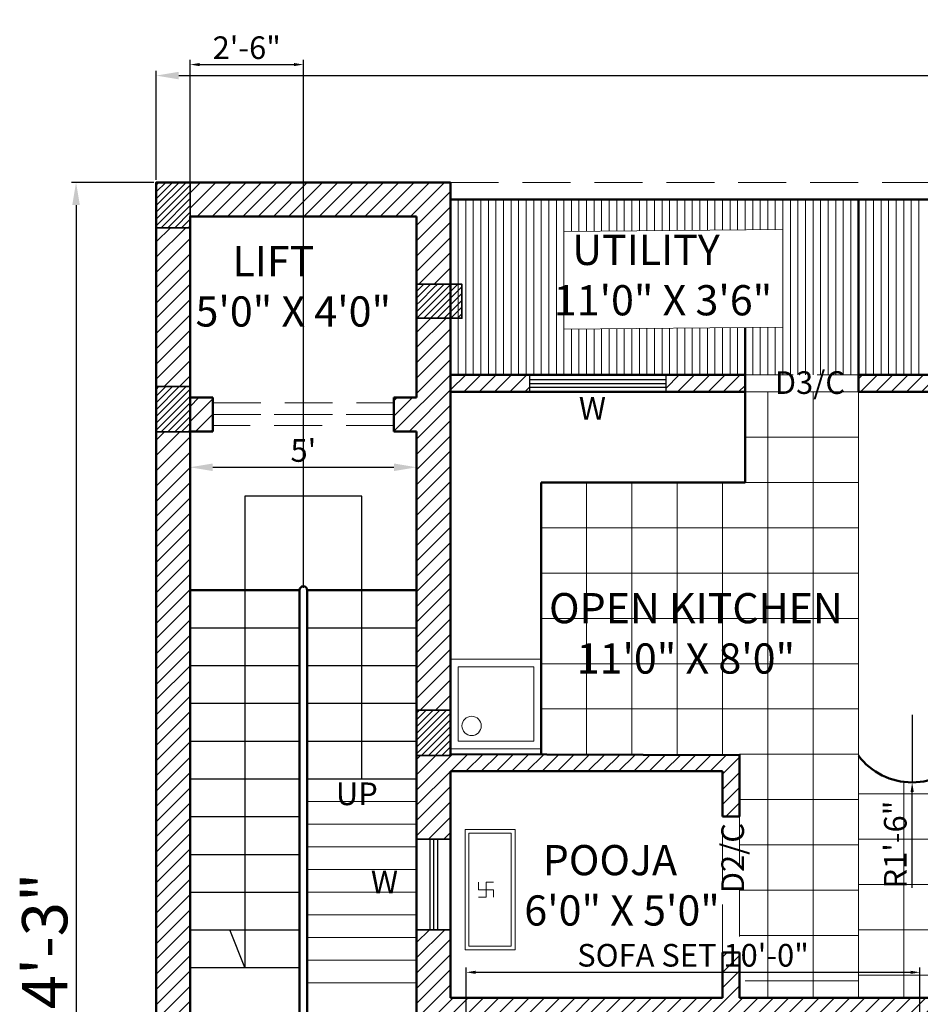
# Model space of a CAD drawing. Units: millimetres. Extents: x 225995 to 227247, y 225507 to 226008.
# Tile 2 of 23: x 225998 to 226236, y 225743 to 226004. Entities that reach past the tile are written whole.
import ezdxf

# ---------------------------------------------------------------- set-up
doc = ezdxf.new("R2010")
doc.units = ezdxf.units.MM
doc.linetypes.add('DASHED', pattern=[19.05, 12.7, -6.35])
for name, color, linetype, lineweight in [('A-ANNO-DIMS', 2, 'Continuous', 18), ('A-ANNO-TEXT', 3, 'Continuous', 18), ('A-AREA-IDEN', 30, 'Continuous', 18), ('A-COLS', 40, 'Continuous', 35), ('A-FLOR-PATT', 8, 'Continuous', 13), ('A-FLOR-STRS', 141, 'Continuous', 25), ('A-FURN', 9, 'Continuous', 18), ('A-GLAZ', 4, 'Continuous', 25), ('A-WALL', 7, 'Continuous', 50), ('A-WALL-OVHD', 1, 'DASHED', 18), ('A-WALL-PATT', 8, 'Continuous', 13)]:
    doc.layers.add(name, color=color, linetype=linetype, lineweight=lineweight)
doc.styles.get("Standard").update_dxf_attribs({"font": 'arial.ttf'})
doc.dimstyles.new('ISO-25', dxfattribs={"dimtxt": 6, "dimasz": 2.5, "dimexe": 1.25, "dimexo": 0.625, "dimtad": 1, "dimdec": 0, "dimlunit": 3, "dimtxsty": 'Standard', "dimcen": 2.5, "dimadec": 0, "dimazin": 0, "dimtfac": 1, "dimtdec": 0, "dimtmove": 0, "dimatfit": 3, "dimfxl": 1, "dimarcsym": 0})
pattern_1 = [(45, (-277.5, 234), (-0.898025612, 0.898025612), [])]

# ---------------------------------------------------------------- blocks, each defined once
blk = doc.blocks.new('*D65')
at = {"layer": 'A-ANNO-DIMS', "color": 0, "lineweight": -2, "transparency": 16777216}
for p, q in [((226042.88, 225884.42), (226042.88, 225886.55)), ((226048.88, 225885.3), (226096.88, 225885.3)), ((226102.88, 225884.42), (226102.88, 225886.55))]:
    blk.add_line(p, q, dxfattribs=at)
at = {"layer": 'A-ANNO-DIMS', "color": 0, "transparency": 16777216}
for points in [[(226048.88, 225886.3), (226048.88, 225884.3), (226042.88, 225885.3)], [(226096.88, 225886.3), (226096.88, 225884.3), (226102.88, 225885.3)]]:
    blk.add_solid(points, dxfattribs=at)
at = {"layer": 'Defpoints', "color": 0, "transparency": 16777216}
for p in [(226102.88, 225885.3), (226042.88, 225883.79), (226102.88, 225883.79)]:
    blk.add_point(p, dxfattribs=at)
at = {"layer": 'A-ANNO-DIMS', "color": 0, "transparency": 16777216, "insert": (226072.88, 225888.97), "char_height": 6, "attachment_point": 5}
blk.add_mtext("5'", dxfattribs=at)
blk = doc.blocks.new('*D68')
at = {"layer": 'A-ANNO-DIMS', "color": 0, "lineweight": -2, "transparency": 16777216}
for p, q in [((226033.88, 225961.4), (226033.88, 225990.31)), ((226039.88, 225989.06), (226559.88, 225989.06)), ((226565.88, 225961.4), (226565.88, 225990.31))]:
    blk.add_line(p, q, dxfattribs=at)
at = {"layer": 'A-ANNO-DIMS', "color": 0, "transparency": 16777216}
for points in [[(226039.88, 225990.06), (226039.88, 225988.06), (226033.88, 225989.06)], [(226559.88, 225990.06), (226559.88, 225988.06), (226565.88, 225989.06)]]:
    blk.add_solid(points, dxfattribs=at)
at = {"layer": 'Defpoints', "color": 0, "transparency": 16777216}
for p in [(226565.88, 225989.06), (226033.88, 225960.77), (226565.88, 225960.77)]:
    blk.add_point(p, dxfattribs=at)
at = {"layer": 'A-ANNO-DIMS', "color": 0, "transparency": 16777216, "insert": (226299.88, 225995.68), "char_height": 12, "attachment_point": 5}
blk.add_mtext('44\'-4"', dxfattribs=at)
blk = doc.blocks.new('*D69')
at = {"layer": 'A-ANNO-DIMS', "color": 0, "lineweight": -2, "transparency": 16777216}
for p, q in [((226033.25, 225960.77), (226011.42, 225960.77)), ((226012.67, 225954.77), (226012.67, 225555.77)), ((226033.25, 225549.77), (226011.42, 225549.77))]:
    blk.add_line(p, q, dxfattribs=at)
at = {"layer": 'A-ANNO-DIMS', "color": 0, "transparency": 16777216}
for points in [[(226011.67, 225954.77), (226013.67, 225954.77), (226012.67, 225960.77)], [(226011.67, 225555.77), (226013.67, 225555.77), (226012.67, 225549.77)]]:
    blk.add_solid(points, dxfattribs=at)
at = {"layer": 'Defpoints', "color": 0, "transparency": 16777216}
for p in [(226033.88, 225960.77), (226012.67, 225549.77), (226033.88, 225549.77)]:
    blk.add_point(p, dxfattribs=at)
at = {"layer": 'A-ANNO-DIMS', "color": 0, "transparency": 16777216, "insert": (226005.92, 225755.27), "char_height": 12, "attachment_point": 5, "rotation": 90}
blk.add_mtext('34\'-3"', dxfattribs=at)
blk = doc.blocks.new('*D83')
at = {"layer": 'A-ANNO-DIMS', "color": 0, "lineweight": -2, "transparency": 16777216}
for p, q in [((226115.99, 225734.11), (226115.99, 225752.77)), ((226118.49, 225751.52), (226233.69, 225751.52)), ((226236.19, 225734.11), (226236.19, 225752.77))]:
    blk.add_line(p, q, dxfattribs=at)
at = {"layer": 'A-ANNO-DIMS', "color": 0, "transparency": 16777216}
for points in [[(226118.49, 225751.93), (226118.49, 225751.1), (226115.99, 225751.52)], [(226233.69, 225751.93), (226233.69, 225751.1), (226236.19, 225751.52)]]:
    blk.add_solid(points, dxfattribs=at)
at = {"layer": 'Defpoints', "color": 0, "transparency": 16777216}
for p in [(226236.19, 225751.52), (226115.99, 225733.49), (226236.19, 225733.49)]:
    blk.add_point(p, dxfattribs=at)
at = {"layer": 'A-ANNO-DIMS', "color": 0, "transparency": 16777216, "insert": (226176.09, 225755.25), "char_height": 6, "attachment_point": 5}
blk.add_mtext('SOFA SET 10\'-0"', dxfattribs=at)
blk = doc.blocks.new('*D112')
at = {"layer": 'A-ANNO-DIMS', "color": 0, "lineweight": -2, "transparency": 16777216}
for p, q in [((226042.88, 225853.4), (226042.88, 225993.22)), ((226045.38, 225991.97), (226070.38, 225991.97)), ((226072.88, 225853.4), (226072.88, 225993.22))]:
    blk.add_line(p, q, dxfattribs=at)
at = {"layer": 'A-ANNO-DIMS', "color": 0, "transparency": 16777216}
for points in [[(226045.38, 225992.39), (226045.38, 225991.56), (226042.88, 225991.97)], [(226070.38, 225992.39), (226070.38, 225991.56), (226072.88, 225991.97)]]:
    blk.add_solid(points, dxfattribs=at)
at = {"layer": 'Defpoints', "color": 0, "transparency": 16777216}
for p in [(226072.88, 225991.97), (226042.88, 225852.77), (226072.88, 225852.77)]:
    blk.add_point(p, dxfattribs=at)
at = {"layer": 'A-ANNO-DIMS', "color": 0, "transparency": 16777216, "insert": (226057.88, 225995.66), "char_height": 6, "attachment_point": 5}
blk.add_mtext('2\'-6"', dxfattribs=at)
blk = doc.blocks.new('*D135')
at = {"layer": 'A-ANNO-DIMS', "color": 0, "lineweight": -2, "transparency": 16777216}
for p, q in [((226234.13, 225819.69), (226234.13, 225801.82)), ((226234.13, 225773.88), (226234.13, 225799.32))]:
    blk.add_line(p, q, dxfattribs=at)
at = {"layer": 'A-ANNO-DIMS', "color": 0, "transparency": 16777216}
blk.add_solid([(226233.71, 225799.32), (226234.54, 225799.32), (226234.13, 225801.82)], dxfattribs=at)
at = {"layer": 'Defpoints', "color": 0, "transparency": 16777216}
for p in [(226234.13, 225819.69), (226234.13, 225801.82)]:
    blk.add_point(p, dxfattribs=at)
at = {"layer": 'A-ANNO-DIMS', "color": 0, "transparency": 16777216, "insert": (226230.44, 225785.35), "char_height": 6, "attachment_point": 5, "rotation": 89.9987}
blk.add_mtext('R1\'-6"', dxfattribs=at)

msp = doc.modelspace()

# ---------------------------------------------------------------- hatches: boundary and pattern name
at = {"layer": 'A-WALL-PATT'}
h = msp.add_hatch(dxfattribs=at)
h.set_pattern_fill('ANSI31', color=256, scale=0.4)
h.set_pattern_definition([(45, (-69, 378), (-0.898025612, 0.898025612), [])])
h.paths.add_polyline_path([(226042.88, 225960.77), (226033.88, 225960.77), (226033.88, 225948.77), (226042.88, 225948.77)])
h = msp.add_hatch(dxfattribs=at)
h.set_pattern_fill('ANSI31', color=256, scale=0.9)
h.paths.add_polyline_path([(226111.88, 225960.77), (226042.88, 225960.77), (226042.88, 225951.77), (226102.88, 225951.77), (226102.88, 225933.77), (226111.88, 225933.77)])
h = msp.add_hatch(dxfattribs=at)
h.set_pattern_fill('ANSI31', color=256, scale=0.9)
h.paths.add_polyline_path([(226042.88, 225948.77), (226033.88, 225948.77), (226033.88, 225906.68), (226042.88, 225906.68)])
h = msp.add_hatch(dxfattribs=at)
h.set_pattern_fill('ANSI31', color=256, scale=0.4)
h.set_pattern_definition(pattern_1)
h.paths.add_polyline_path([(226107.38, 225933.77), (226102.88, 225933.77), (226102.88, 225929.27), (226107.38, 225929.27)])
h = msp.add_hatch(dxfattribs=at)
h.set_pattern_fill('ANSI31', color=256, scale=0.4)
h.set_pattern_definition(pattern_1)
h.paths.add_polyline_path([(226114.88, 225933.77), (226107.38, 225933.77), (226107.38, 225929.27), (226114.88, 225929.27)])
h = msp.add_hatch(dxfattribs=at)
h.set_pattern_fill('ANSI31', color=256, scale=0.4)
h.set_pattern_definition(pattern_1)
h.paths.add_polyline_path([(226107.38, 225929.27), (226102.88, 225929.27), (226102.88, 225924.77), (226107.38, 225924.77)])
h = msp.add_hatch(dxfattribs=at)
h.set_pattern_fill('ANSI31', color=256, scale=0.4)
h.set_pattern_definition(pattern_1)
h.paths.add_polyline_path([(226114.88, 225929.27), (226107.38, 225929.27), (226107.38, 225924.77), (226114.88, 225924.77)])
h = msp.add_hatch(dxfattribs=at)
h.set_pattern_fill('ANSI31', color=256, scale=0.9)
h.paths.add_polyline_path([(226111.88, 225924.77), (226102.88, 225924.77), (226102.88, 225903.77), (226096.88, 225903.77), (226096.88, 225894.77), (226102.88, 225894.77), (226102.88, 225820.92), (226111.88, 225820.92)])
h = msp.add_hatch(dxfattribs=at)
h.set_pattern_fill('ANSI31', color=256, scale=0.9)
h.paths.add_polyline_path([(226248.38, 225924.77), (226243.88, 225924.77), (226243.88, 225909.77), (226219.88, 225909.77), (226219.88, 225905.27), (226243.88, 225905.27), (226244.03, 225817.91), (226248.38, 225817.91)])
h = msp.add_hatch(dxfattribs=at)
h.set_pattern_fill('ANSI31', color=256, scale=0.9)
h.paths.add_polyline_path([(226132.88, 225909.77), (226111.88, 225909.77), (226111.88, 225905.27), (226132.88, 225905.27)])
h = msp.add_hatch(dxfattribs=at)
h.set_pattern_fill('ANSI31', color=256, scale=0.9)
h.paths.add_polyline_path([(226189.88, 225909.77), (226168.88, 225909.77), (226168.88, 225905.27), (226189.88, 225905.27)])
h = msp.add_hatch(dxfattribs=at)
h.set_pattern_fill('ANSI31', color=256, scale=0.4)
h.set_pattern_definition([(45, (-69, 323.9086), (-0.898025612, 0.898025612), [])])
h.paths.add_polyline_path([(226042.88, 225906.68), (226033.88, 225906.68), (226033.88, 225894.68), (226042.88, 225894.68)])
h = msp.add_hatch(dxfattribs=at)
h.set_pattern_fill('ANSI31', color=256, scale=0.9)
h.paths.add_polyline_path([(226048.88, 225903.77), (226042.88, 225903.77), (226042.88, 225894.77), (226048.88, 225894.77)])
h = msp.add_hatch(dxfattribs=at)
h.set_pattern_fill('ANSI31', color=256, scale=0.9)
h.paths.add_polyline_path([(226042.88, 225894.68), (226033.88, 225894.68), (226033.88, 225708.42), (226042.88, 225708.42)])
h = msp.add_hatch(dxfattribs=at)
h.set_pattern_fill('ANSI31', color=256, scale=0.4)
h.set_pattern_definition([(45, (4e-05, 238.1468), (-0.898025612, 0.898025612), [])])
h.paths.add_polyline_path([(226111.88, 225820.92), (226102.88, 225820.92), (226102.88, 225808.92), (226111.88, 225808.92)])
h = msp.add_hatch(dxfattribs=at)
h.set_pattern_fill('ANSI31', color=256, scale=0.9)
h.paths.add_polyline_path([(226188.38, 225809.07), (226111.88, 225809.27), (226111.88, 225808.92), (226102.88, 225808.92), (226102.88, 225786.77), (226111.88, 225786.77), (226111.88, 225804.77), (226183.88, 225804.77), (226183.88, 225792.77), (226188.38, 225792.77)])
h = msp.add_hatch(dxfattribs=at)
h.set_pattern_fill('ANSI31', color=256, scale=0.9)
h.paths.add_polyline_path([(226111.88, 225740.27), (226248.38, 225740.27), (226248.38, 225744.77), (226188.38, 225744.77), (226188.38, 225756.77), (226183.88, 225756.77), (226183.88, 225744.77), (226111.88, 225744.77), (226111.88, 225762.77), (226102.88, 225762.77), (226102.88, 225702.77), (226111.88, 225702.77)])

# ---------------------------------------------------------------- linework, layer by layer
at = {"layer": 'A-ANNO-TEXT'}
msp.add_lwpolyline([(226141.88, 225947.73), (226199.88, 225948.29), (226199.88, 225922.41), (226141.88, 225921.84)], close=True, dxfattribs=at)
at = {"layer": 'A-COLS'}
for p, q in [((226111.88, 225786.77), (226102.88, 225786.77)), ((226111.88, 225762.77), (226102.88, 225762.77))]:
    msp.add_line(p, q, dxfattribs=at)
for points in [[(226042.88, 225948.77), (226033.88, 225948.77), (226033.88, 225960.77), (226042.88, 225960.77)], [(226102.88, 225924.77), (226102.88, 225933.77), (226114.88, 225933.77), (226114.88, 225924.77)], [(226042.88, 225894.68), (226033.88, 225894.68), (226033.88, 225906.68), (226042.88, 225906.68)], [(226111.88, 225808.92), (226102.88, 225808.92), (226102.88, 225820.92), (226111.88, 225820.92)]]:
    msp.add_lwpolyline(points, close=True, dxfattribs=at)
at = {"layer": 'A-FLOR-PATT'}
for p, q in [((226195.88, 225744.77), (226195.88, 225905.27)), ((226207.88, 225744.77), (226207.88, 225905.27)), ((226219.88, 225744.77), (226219.88, 225905.27)), ((226189.88, 225893.27), (226219.88, 225893.27)), ((226147.88, 225809.27), (226147.88, 225881.27)), ((226159.88, 225809.27), (226159.88, 225881.27)), ((226171.88, 225809.27), (226171.88, 225881.27)), ((226183.88, 225809.27), (226183.88, 225881.27)), ((226189.88, 225881.27), (226219.88, 225881.27)), ((226135.88, 225869.27), (226219.88, 225869.27)), ((226135.88, 225857.27), (226219.88, 225857.27)), ((226135.88, 225845.27), (226219.88, 225845.27)), ((226135.88, 225833.27), (226219.88, 225833.27)), ((226135.88, 225821.27), (226219.88, 225821.27)), ((226188.38, 225809.27), (226219.88, 225809.27)), ((226231.88, 225744.77), (226231.88, 225801.96)), ((226219.88, 225798.77), (226380.38, 225798.77)), ((226102.88, 225796.77), (226073.88, 225796.77)), ((226188.38, 225797.27), (226219.88, 225797.27)), ((226102.88, 225790.77), (226073.88, 225790.77)), ((226188.38, 225785.27), (226219.88, 225785.27)), ((226219.88, 225786.77), (226380.38, 225786.77)), ((226102.88, 225784.77), (226073.88, 225784.77)), ((226102.88, 225778.77), (226073.88, 225778.77)), ((226219.88, 225774.77), (226380.38, 225774.77)), ((226102.88, 225772.77), (226073.88, 225772.77)), ((226188.38, 225773.27), (226219.88, 225773.27)), ((226102.88, 225766.77), (226073.88, 225766.77)), ((226219.88, 225762.77), (226380.38, 225762.77)), ((226102.88, 225760.77), (226073.88, 225760.77)), ((226188.38, 225761.27), (226219.88, 225761.27)), ((226102.88, 225754.77), (226073.88, 225754.77)), ((226102.88, 225748.77), (226073.88, 225748.77)), ((226189.88, 225749.27), (226219.88, 225749.27)), ((226219.88, 225750.77), (226380.38, 225750.77))]:
    msp.add_line(p, q, dxfattribs=at)
at = {"layer": 'A-FLOR-STRS'}
for p, q in [((226088.38, 225877.62), (226057.38, 225877.62)), ((226057.38, 225877.62), (226057.38, 225752.77)), ((226088.38, 225802.77), (226088.38, 225877.62)), ((226042.88, 225842.77), (226071.88, 225842.77)), ((226073.88, 225842.77), (226102.88, 225842.77)), ((226042.88, 225832.77), (226071.88, 225832.77)), ((226073.88, 225832.77), (226102.88, 225832.77)), ((226042.88, 225822.77), (226071.88, 225822.77)), ((226073.88, 225822.77), (226102.88, 225822.77)), ((226042.88, 225812.77), (226071.88, 225812.77)), ((226073.88, 225812.77), (226102.88, 225812.77)), ((226042.88, 225802.77), (226071.88, 225802.77)), ((226073.88, 225802.77), (226102.88, 225802.77)), ((226042.88, 225792.77), (226071.88, 225792.77)), ((226042.88, 225782.77), (226071.88, 225782.77)), ((226042.88, 225772.77), (226071.88, 225772.77)), ((226042.88, 225762.77), (226071.88, 225762.77)), ((226057.38, 225752.77), (226053.39, 225762.77)), ((226053.39, 225762.77), (226057.38, 225762.77)), ((226042.88, 225752.77), (226071.88, 225752.77))]:
    msp.add_line(p, q, dxfattribs=at)
at = {"layer": 'A-FURN'}
for p, q in [((226113.88, 225909.77), (226113.88, 225956.27)), ((226115.88, 225909.77), (226115.88, 225956.27)), ((226117.88, 225909.77), (226117.88, 225956.27)), ((226119.88, 225909.77), (226119.88, 225956.27)), ((226119.88, 225909.77), (226119.88, 225956.27)), ((226121.88, 225909.77), (226121.88, 225956.27)), ((226123.88, 225909.77), (226123.88, 225956.27)), ((226125.88, 225909.77), (226125.88, 225956.27)), ((226127.88, 225909.77), (226127.88, 225956.27)), ((226129.88, 225909.77), (226129.88, 225956.27)), ((226131.88, 225909.77), (226131.88, 225956.27)), ((226133.88, 225909.77), (226133.88, 225956.27)), ((226135.88, 225909.77), (226135.88, 225956.27)), ((226137.88, 225909.77), (226137.88, 225956.27)), ((226139.88, 225909.77), (226139.88, 225956.27)), ((226141.88, 225909.77), (226141.88, 225956.27)), ((226143.88, 225947.75), (226143.88, 225956.27)), ((226145.88, 225947.76), (226145.88, 225956.27)), ((226147.88, 225947.78), (226147.88, 225956.27)), ((226149.88, 225947.8), (226149.88, 225956.27)), ((226151.88, 225947.82), (226151.88, 225956.27)), ((226153.88, 225947.84), (226153.88, 225956.27)), ((226155.88, 225947.86), (226155.88, 225956.27)), ((226157.88, 225947.88), (226157.88, 225956.27)), ((226159.88, 225947.9), (226159.88, 225956.27)), ((226161.88, 225947.92), (226161.88, 225956.27)), ((226163.88, 225947.94), (226163.88, 225956.27)), ((226165.88, 225947.96), (226165.88, 225956.27)), ((226167.88, 225947.98), (226167.88, 225956.27)), ((226169.88, 225948), (226169.88, 225956.27)), ((226171.88, 225948.02), (226171.88, 225956.27)), ((226173.88, 225948.04), (226173.88, 225956.27)), ((226175.88, 225948.06), (226175.88, 225956.27)), ((226177.88, 225948.08), (226177.88, 225956.27)), ((226179.88, 225948.1), (226179.88, 225956.27)), ((226181.88, 225948.12), (226181.88, 225956.27)), ((226183.88, 225948.14), (226183.88, 225956.27)), ((226185.88, 225948.15), (226185.88, 225956.27)), ((226187.88, 225948.17), (226187.88, 225956.27)), ((226189.88, 225948.19), (226189.88, 225956.27)), ((226191.88, 225948.21), (226191.88, 225956.27)), ((226193.88, 225948.23), (226193.88, 225956.27)), ((226195.88, 225948.25), (226195.88, 225956.27)), ((226197.88, 225948.27), (226197.88, 225956.27)), ((226199.88, 225909.77), (226199.88, 225956.27)), ((226201.88, 225909.77), (226201.88, 225956.27)), ((226203.88, 225909.77), (226203.88, 225956.27)), ((226205.88, 225909.77), (226205.88, 225956.27)), ((226207.88, 225909.77), (226207.88, 225956.27)), ((226209.88, 225909.77), (226209.88, 225956.27)), ((226211.88, 225909.77), (226211.88, 225956.27)), ((226213.88, 225909.77), (226213.88, 225956.27)), ((226215.88, 225909.77), (226215.88, 225956.27)), ((226217.88, 225909.77), (226217.88, 225956.27)), ((226221.88, 225909.77), (226221.88, 225956.27)), ((226223.88, 225909.77), (226223.88, 225956.27)), ((226225.88, 225909.77), (226225.88, 225956.27)), ((226227.88, 225909.77), (226227.88, 225956.27)), ((226229.88, 225909.77), (226229.88, 225956.27)), ((226231.88, 225909.77), (226231.88, 225956.27)), ((226233.88, 225909.77), (226233.88, 225956.27)), ((226235.88, 225909.77), (226235.88, 225956.27)), ((226143.88, 225909.77), (226143.88, 225921.86)), ((226145.88, 225909.77), (226145.88, 225921.88)), ((226147.88, 225909.77), (226147.88, 225921.9)), ((226149.88, 225909.77), (226149.88, 225921.92)), ((226151.88, 225909.77), (226151.88, 225921.94)), ((226153.88, 225909.77), (226153.88, 225921.96)), ((226155.88, 225909.77), (226155.88, 225921.98)), ((226157.88, 225909.77), (226157.88, 225922)), ((226159.88, 225909.77), (226159.88, 225922.02)), ((226161.88, 225909.77), (226161.88, 225922.04)), ((226163.88, 225909.77), (226163.88, 225922.06)), ((226165.88, 225909.77), (226165.88, 225922.07)), ((226167.88, 225909.77), (226167.88, 225922.09)), ((226169.88, 225909.77), (226169.88, 225922.11)), ((226171.88, 225909.77), (226171.88, 225922.13)), ((226173.88, 225909.77), (226173.88, 225922.15)), ((226175.88, 225909.77), (226175.88, 225922.17)), ((226177.88, 225909.77), (226177.88, 225922.19)), ((226179.88, 225909.77), (226179.88, 225922.21)), ((226181.88, 225909.77), (226181.88, 225922.23)), ((226183.88, 225909.77), (226183.88, 225922.25)), ((226185.88, 225909.77), (226185.88, 225922.27)), ((226187.88, 225909.77), (226187.88, 225922.29)), ((226191.88, 225909.77), (226191.88, 225922.33)), ((226193.88, 225909.77), (226193.88, 225922.35)), ((226195.88, 225909.77), (226195.88, 225922.37)), ((226197.88, 225909.77), (226197.88, 225922.39)), ((226132.88, 225909.77), (226132.88, 225905.27)), ((226168.88, 225909.77), (226168.88, 225905.27)), ((226119.25, 225773.41), (226119.25, 225775.41)), ((226121.25, 225771.41), (226121.25, 225775.41)), ((226121.25, 225775.41), (226123.25, 225775.41)), ((226119.25, 225773.41), (226123.25, 225773.41)), ((226123.25, 225773.41), (226123.25, 225771.41)), ((226121.25, 225771.41), (226119.25, 225771.41))]:
    msp.add_line(p, q, dxfattribs=at)
for points in [[(226111.88, 225834.44), (226135.88, 225834.44), (226135.88, 225810.75), (226111.88, 225810.75)], [(226113.88, 225832.44), (226133.88, 225832.44), (226133.88, 225812.75), (226113.88, 225812.75)], [(226115.73, 225789.39), (226128.93, 225789.39), (226128.93, 225757.43), (226115.73, 225757.43)], [(226116.73, 225788.39), (226127.93, 225788.39), (226127.93, 225758.43), (226116.73, 225758.43)]]:
    msp.add_lwpolyline(points, close=True, dxfattribs=at)
msp.add_circle((226117.44, 225816.79), 2.56, dxfattribs=at)
at = {"layer": 'A-GLAZ'}
for p, q in [((226132.88, 225908.52), (226168.88, 225908.52)), ((226132.88, 225907.52), (226168.88, 225907.52)), ((226132.88, 225906.52), (226168.88, 225906.52)), ((226106.38, 225786.77), (226106.38, 225762.77)), ((226107.38, 225786.77), (226107.38, 225762.77)), ((226108.38, 225786.77), (226108.38, 225762.77))]:
    msp.add_line(p, q, dxfattribs=at)
for points in [[(226132.88, 225909.77), (226168.88, 225909.77), (226168.88, 225905.27), (226132.88, 225905.27)], [(226102.88, 225786.77), (226111.88, 225786.77), (226111.88, 225762.77), (226102.88, 225762.77)]]:
    msp.add_lwpolyline(points, close=True, dxfattribs=at)
at = {"layer": 'A-WALL'}
for p, q in [((226033.88, 225672.77), (226033.88, 225960.77)), ((226111.88, 225960.77), (226033.88, 225960.77)), ((226033.88, 225960.77), (226033.88, 225672.77)), ((226033.88, 225960.77), (226111.88, 225960.77)), ((226111.88, 225809.27), (226111.88, 225960.77)), ((226111.88, 225909.77), (226111.88, 225960.77)), ((226111.88, 225960.77), (226111.88, 225956.27)), ((226111.88, 225956.27), (226239.38, 225956.27)), ((226219.88, 225909.77), (226219.88, 225956.27)), ((226042.88, 225951.77), (226102.88, 225951.77)), ((226042.88, 225903.77), (226042.88, 225951.77)), ((226042.88, 225672.77), (226042.88, 225951.77)), ((226042.88, 225951.77), (226102.88, 225951.77)), ((226102.88, 225903.77), (226102.88, 225951.77)), ((226102.88, 225951.77), (226102.88, 225903.77)), ((226189.88, 225909.77), (226189.88, 225922.31)), ((226111.88, 225909.77), (226189.88, 225909.77)), ((226189.88, 225909.77), (226111.88, 225909.77)), ((226189.88, 225905.27), (226189.88, 225909.77)), ((226189.88, 225905.27), (226189.88, 225909.77)), ((226219.88, 225905.27), (226219.88, 225909.77)), ((226219.88, 225909.77), (226243.88, 225909.77)), ((226219.88, 225905.27), (226219.88, 225909.77)), ((226219.88, 225909.77), (226243.88, 225909.77)), ((226111.88, 225905.27), (226189.88, 225905.27)), ((226111.88, 225809.27), (226111.88, 225905.27)), ((226111.88, 225905.27), (226189.88, 225905.27)), ((226189.88, 225905.27), (226189.88, 225881.27)), ((226219.88, 225905.27), (226243.88, 225905.27)), ((226243.88, 225905.27), (226219.88, 225905.27)), ((226042.88, 225903.77), (226048.88, 225903.77)), ((226048.88, 225903.77), (226048.88, 225894.77)), ((226096.88, 225903.77), (226096.88, 225894.77)), ((226096.88, 225903.77), (226102.88, 225903.77)), ((226102.88, 225903.77), (226096.88, 225903.77)), ((226096.88, 225903.77), (226096.88, 225894.77)), ((226042.88, 225672.77), (226042.88, 225894.77)), ((226042.88, 225894.77), (226048.88, 225894.77)), ((226096.88, 225894.77), (226102.88, 225894.77)), ((226096.88, 225894.77), (226102.88, 225894.77)), ((226102.88, 225660.77), (226102.88, 225894.77)), ((226102.88, 225894.77), (226102.88, 225660.77)), ((226135.88, 225881.27), (226189.88, 225881.27)), ((226135.88, 225809.27), (226135.88, 225881.27)), ((226042.88, 225852.77), (226071.88, 225852.77)), ((226071.88, 225852.77), (226071.88, 225672.77)), ((226073.88, 225852.77), (226073.88, 225672.77)), ((226073.88, 225852.77), (226102.88, 225852.77)), ((226111.88, 225809.27), (226188.38, 225809.07)), ((226188.42, 225809.07), (226111.88, 225809.27)), ((226188.38, 225792.77), (226188.38, 225809.27)), ((226188.38, 225792.77), (226188.42, 225809.07)), ((226111.88, 225804.77), (226183.88, 225804.77)), ((226111.88, 225744.77), (226111.88, 225804.77)), ((226111.88, 225744.77), (226111.88, 225804.77)), ((226111.88, 225804.77), (226183.88, 225804.77)), ((226183.88, 225792.77), (226183.88, 225804.77)), ((226183.88, 225804.77), (226183.88, 225792.77)), ((226183.88, 225792.77), (226188.38, 225792.77)), ((226183.88, 225792.77), (226188.38, 225792.77)), ((226183.88, 225744.77), (226183.88, 225756.77)), ((226183.88, 225756.77), (226188.38, 225756.77)), ((226188.38, 225756.77), (226183.88, 225756.77)), ((226183.88, 225756.77), (226183.88, 225744.77)), ((226188.38, 225744.77), (226188.38, 225756.77)), ((226188.38, 225744.77), (226188.38, 225756.77)), ((226111.88, 225744.77), (226183.88, 225744.77)), ((226183.88, 225744.77), (226111.88, 225744.77)), ((226188.38, 225744.77), (226248.38, 225744.77)), ((226248.38, 225744.77), (226188.38, 225744.77))]:
    msp.add_line(p, q, dxfattribs=at)
for centre, radius, start, end in [((226072.88, 225852.77), 1, 0, 180), ((226234.13, 225819.69), 17.87, 217.0967, 322.9033)]:
    msp.add_arc(centre, radius, start, end, dxfattribs=at)
at = {"layer": 'A-WALL-OVHD'}
for p, q in [((226111.88, 225960.77), (226243.88, 225960.77)), ((226111.88, 225956.27), (226239.38, 225956.27))]:
    msp.add_line(p, q, dxfattribs=at)
for points in [[(226189.88, 225909.77), (226219.88, 225909.77), (226219.88, 225905.27), (226189.88, 225905.27)], [(226048.88, 225902.41), (226096.88, 225902.41), (226096.88, 225896.34), (226048.88, 225896.34)], [(226048.88, 225899.27), (226096.88, 225899.27), (226096.88, 225899.27), (226048.88, 225899.27)], [(226183.88, 225792.77), (226188.38, 225792.77), (226188.38, 225756.77), (226183.88, 225756.77)]]:
    msp.add_lwpolyline(points, close=True, dxfattribs=at)

# ---------------------------------------------------------------- texts
at = {"layer": 'A-ANNO-TEXT', "char_height": 6, "attachment_point": 1}
for s, insert in [('D3/C', (226197.74, 225910.73)), ('   W', (226140.34, 225903.91)), ('   UP', (226076, 225801.8)), ('   W', (226085.26, 225778.45))]:
    msp.add_mtext_dynamic_manual_height_columns(s, width=24.8115, gutter_width=12.5, heights=[0], dxfattribs=dict(at, insert=insert))
at = {"layer": 'A-ANNO-TEXT', "insert": (226183.59, 225772.46), "char_height": 6, "attachment_point": 1, "rotation": 90}
msp.add_mtext_dynamic_manual_height_columns('D2/C', width=8.157, gutter_width=12.5, heights=[0], dxfattribs=at)
at = {"layer": 'A-AREA-IDEN', "char_height": 8, "attachment_point": 1}
for s, heights, insert in [('     UTILITY \\P   11\'0" X 3\'6"', [21.51], (226131.88, 225946.88)), ('       LIFT\\P   5\'0" X 4\'0"', [0], (226036.98, 225943.91)), ('OPEN KITCHEN\\P   11\'0" X 8\'0"', [0], (226137.94, 225851.98)), ('     POOJA\\P   6\'0" X 5\'0"', [0], (226124.06, 225785.24))]:
    msp.add_mtext_dynamic_manual_height_columns(s, width=85.4795, gutter_width=12.5, heights=heights, dxfattribs=dict(at, insert=insert))

# ---------------------------------------------------------------- dimensions: what is measured, and where the dimension line sits
at = {"layer": 'A-ANNO-DIMS'}
for base, p1, p2, override, picture, middle in [((226565.88, 225989.06), (226033.88, 225960.77), (226565.88, 225960.77), {"dimtxt": 12, "dimasz": 6, "dimclrd": 0, "dimclre": 0, "dimclrt": 0}, '*D68', (226299.88, 225995.68)), ((226072.88, 225991.97), (226042.88, 225852.77), (226072.88, 225852.77), {"dimdec": 1, "dimlfac": 1, "dimrnd": 0, "dimzin": 1, "dimdsep": 46, "dimlunit": 4, "dimfrac": 2}, '*D112', (226057.88, 225995.66)), ((226102.88, 225885.3), (226042.88, 225883.79), (226102.88, 225883.79), {"dimtxt": 6, "dimasz": 6, "dimclrd": 0, "dimclre": 0, "dimclrt": 0}, '*D65', (226072.88, 225888.97))]:
    dim = msp.add_linear_dim(base=base, p1=p1, p2=p2, dimstyle='ISO-25', override=override, dxfattribs=at)
    dim.commit()
    dim.dimension.update_dxf_attribs({"geometry": picture, "text_midpoint": middle})
dim = msp.add_linear_dim(base=(226012.67, 225549.77), p1=(226033.88, 225960.77), p2=(226033.88, 225549.77), angle=90, dimstyle='ISO-25', override={"dimtxt": 12, "dimasz": 6, "dimclrd": 0, "dimclre": 0, "dimclrt": 0}, dxfattribs=at)
dim.commit()
dim.dimension.update_dxf_attribs({"geometry": '*D69', "text_midpoint": (226005.92, 225755.27)})
dim = msp.add_radius_dim(center=(226234.13, 225819.69), mpoint=(226234.13, 225801.82), dimstyle='ISO-25', override={"dimdec": 1, "dimlfac": 1, "dimrnd": 0, "dimzin": 1, "dimdsep": 46, "dimlunit": 4, "dimfrac": 2}, dxfattribs=at)
dim.commit()
dim.dimension.update_dxf_attribs({"geometry": '*D135', "text_midpoint": (226230.44, 225785.35)})
dim = msp.add_linear_dim(base=(226236.19, 225751.52), p1=(226115.99, 225733.49), p2=(226236.19, 225733.49), text='SOFA SET <>', dimstyle='ISO-25', override={"dimdec": 1, "dimrnd": 0, "dimzin": 1, "dimlunit": 4, "dimfrac": 2}, dxfattribs=at)
dim.commit()
dim.dimension.update_dxf_attribs({"geometry": '*D83', "text_midpoint": (226176.09, 225755.25)})

doc.saveas('drawing.dxf')
